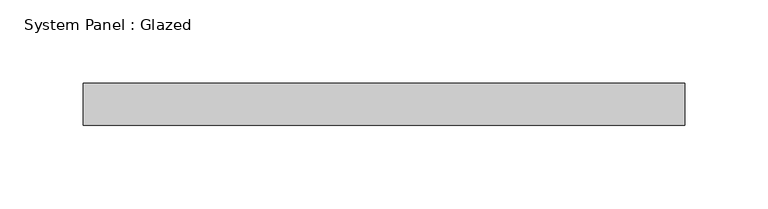
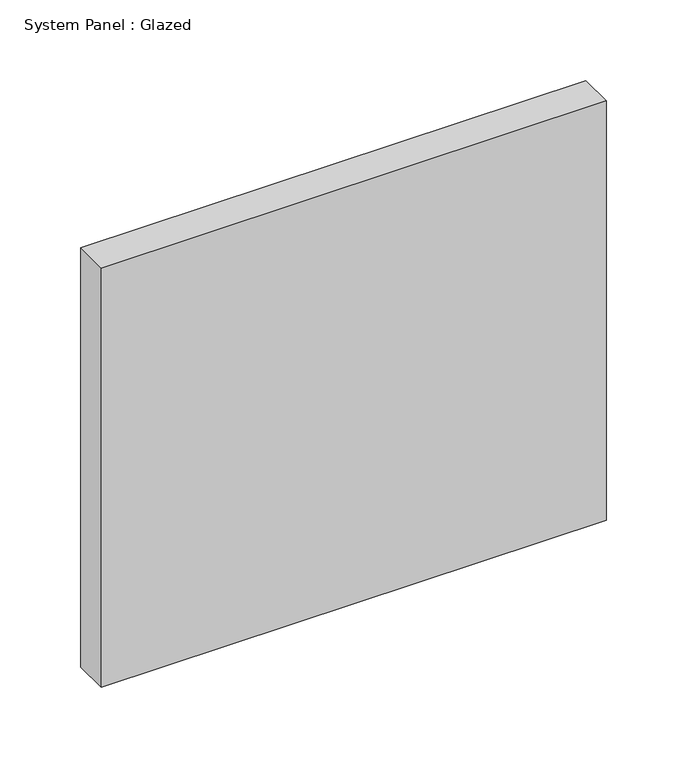
"""IFC4 building model written with IfcOpenShell, lengths in millimetres: plate geometry, System Panel : Glazed."""

from ifc_helpers import new_model, si_unit, origin, origin_with_axes, place, context, project, spatial, polyline, outline, extrude, source, transform, mapped, element, save


def system_panel_glazed_c76c6b52(model_context):
    return source(origin(), model_context, "Body", "SweptSolid", [
        extrude(outline(polyline([(180.975, 19.05), (-180.975, 19.05), (-180.975, 44.45), (180.975, 44.45), (180.975, 19.05)])), origin_with_axes(), (0.0, 0.0, 1.0), 317.5),
    ])


if __name__ == "__main__":
    model = new_model("IFC4")
    model_context = context("Model", 3, world=origin())
    ifc_project = project(units=[si_unit("LENGTHUNIT", "METRE", prefix="MILLI")], contexts=[model_context])
    site = spatial("IfcSite", under=ifc_project)
    building = spatial("IfcBuilding", under=site)
    placement = place(None, origin())
    system_panel_glazed_shape = system_panel_glazed_c76c6b52(model_context)
    element("IfcPlate", 1, ObjectType="System Panel : Glazed", at=placement, inside=building, context=model_context, shape_type="MappedRepresentation", body=[
        mapped(system_panel_glazed_shape, transform((0.0, 0.0, 0.0), x_axis=(1.0, 0.0, 0.0), y_axis=(0.0, 1.0, 0.0), z_axis=(0.0, 0.0, 1.0))),
    ])
    save(model, "model.ifc")

# Revit data of these elements
# Type "System Panel : Glazed"
#   Construction Type Id = "GSP4R"
#   Analytic Construction = "1/8 in Pilkington single glazing"
#   Visual Light Transmittance = 0.9
#   Solar Heat Gain Coefficient = 0.86
#   Heat Transfer Coefficient (U) = 1.18115 BTU/(h·ft²·°F)
#   Define Thermal Properties by = 1
# Element 1 (IfcPlate, "System Panel : Glazed")
#   Materials on its faces: "Glass"
# Materials
#   "Glass": class "Glass", colour RGB 0 128 192, transparency 0.75, Description = "Soda Lime Glass", Cost = 0
